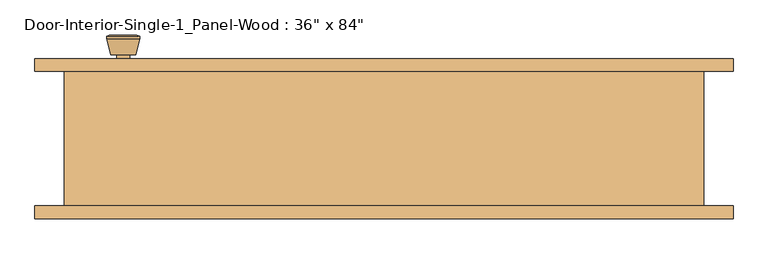
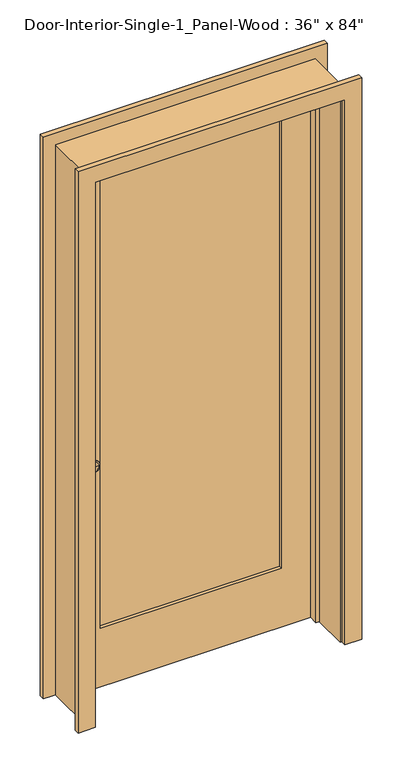
"""IFC4 building model written with IfcOpenShell, lengths in millimetres: door geometry."""

from ifc_helpers import new_model, si_unit, point, frame, frame_2d, origin, place, context, project, spatial, polyline, circle_curve, trimmed, segment, composite_curve, outline, extrude, faceted_brep, source, transform, mapped, element, save
from ifc_brep_helpers import plane_surface, cylinder_surface, revolved_surface, advanced_brep


def door_9c4ddfbd(model_context):
    return source(origin(), model_context, "Body", "SolidModel", [
        advanced_brep(
        [(-393.7, 57.5, 914.4), (-383.7, 57.5, 914.4), (-403.7, 57.5, 914.4), (-373.2241324, 8.5, 914.4), (-393.7, 8.5, 914.4), (-414.1758676, 8.5, 914.4), (-368.7, 10.3278681, 914.4), (-418.7, 10.3278681, 914.4), (-368.7, 13.7915463, 914.4), (-418.7, 13.7915463, 914.4), (-375.063764, 38.5, 914.4), (-412.336236, 38.5, 914.4), (-383.7, 38.5, 914.4), (-403.7, 38.5, 914.4)],
        [
            (0, 1),
            (1, 2, circle_curve(frame((-393.7, 57.5, 914.4), z_axis=(0.0, 1.0, 0.0), x_axis=(-1.0, 0.0, 0.0)), 10.0)),
            (2, 0),
            (2, 1, circle_curve(frame((-393.7, 57.5, 914.4), z_axis=(0.0, 1.0, 0.0), x_axis=(-1.0, 0.0, 0.0)), 10.0)),
            (3, 4),
            (4, 5),
            (5, 3, circle_curve(frame((-393.7, 8.5, 914.4), z_axis=(0.0, -1.0, 0.0), x_axis=(-1.0, 0.0, 0.0)), 20.4758676)),
            (3, 5, circle_curve(frame((-393.7, 8.5, 914.4), z_axis=(0.0, -1.0, 0.0), x_axis=(-1.0, 0.0, 0.0)), 20.4758676)),
            (6, 3),
            (5, 7),
            (7, 6, circle_curve(frame((-393.7, 10.3278681, 914.4), z_axis=(0.0, -1.0, 0.0), x_axis=(-1.0, 0.0, 0.0)), 25.0)),
            (6, 7, circle_curve(frame((-393.7, 10.3278681, 914.4), z_axis=(0.0, -1.0, 0.0), x_axis=(-1.0, 0.0, 0.0)), 25.0)),
            (8, 6),
            (7, 9),
            (9, 8, circle_curve(frame((-393.7, 13.7915463, 914.4), z_axis=(0.0, -1.0, 0.0), x_axis=(-1.0, 0.0, 0.0)), 25.0)),
            (8, 9, circle_curve(frame((-393.7, 13.7915463, 914.4), z_axis=(0.0, -1.0, 0.0), x_axis=(-1.0, 0.0, 0.0)), 25.0)),
            (10, 8),
            (9, 11),
            (11, 10, circle_curve(frame((-393.7, 38.5, 914.4), z_axis=(0.0, -1.0, 0.0), x_axis=(-1.0, 0.0, 0.0)), 18.636236)),
            (10, 11, circle_curve(frame((-393.7, 38.5, 914.4), z_axis=(0.0, -1.0, 0.0), x_axis=(-1.0, 0.0, 0.0)), 18.636236)),
            (12, 10),
            (11, 13),
            (13, 12, circle_curve(frame((-393.7, 38.5, 914.4), z_axis=(0.0, -1.0, 0.0), x_axis=(-1.0, 0.0, 0.0)), 10.0)),
            (12, 13, circle_curve(frame((-393.7, 38.5, 914.4), z_axis=(0.0, -1.0, 0.0), x_axis=(-1.0, 0.0, 0.0)), 10.0)),
            (1, 12),
            (13, 2),
        ],
        [
            plane_surface(frame((-393.7, 57.5, 914.4), z_axis=(0.0, 1.0, 0.0), x_axis=(-1.0, 0.0, 0.0))),
            plane_surface(frame((-393.7, 8.5, 914.4), z_axis=(0.0, -1.0, 0.0), x_axis=(-1.0, 0.0, 0.0))),
            revolved_surface(polyline([(-414.1758676, 8.5, 914.4), (-418.7, 10.3278681, 914.4)]), (-393.7, 57.5, 914.4), (0.0, 1.0, 0.0)),
            cylinder_surface(frame((-393.7, 57.5, 914.4), z_axis=(0.0, 1.0, 0.0), x_axis=(-1.0, 0.0, 0.0)), 25.0),
            revolved_surface(polyline([(-418.7, 13.7915463, 914.4), (-412.336236, 38.5, 914.4)]), (-393.7, 57.5, 914.4), (0.0, 1.0, 0.0)),
            plane_surface(frame((-393.7, 38.5, 914.4), z_axis=(0.0, 1.0, 0.0), x_axis=(-1.0, 0.0, 0.0))),
            cylinder_surface(frame((-393.7, 57.5, 914.4), z_axis=(0.0, 1.0, 0.0), x_axis=(-1.0, 0.0, 0.0)), 10.0),
        ],
        [
            (0, [[1, 2, 3]]),
            (0, [[-3, 4, -1]]),
            (1, [[5, 6, 7]]),
            (1, [[-6, -5, 8]]),
            (2, [[9, -7, 10, 11]]),
            (2, [[-10, -8, -9, 12]]),
            (3, [[13, -11, 14, 15]]),
            (3, [[-14, -12, -13, 16]]),
            (4, [[17, -15, 18, 19]]),
            (4, [[-18, -16, -17, 20]]),
            (5, [[21, -19, 22, 23]]),
            (5, [[-22, -20, -21, 24]]),
            (6, [[25, -23, 26, -2]]),
            (6, [[-26, -24, -25, -4]]),
        ],
    ),
        extrude(outline(composite_curve([segment(trimmed(circle_curve(frame_2d((914.4, -393.7)), 30.0), [point((914.4, -423.7))], [point((914.4, -363.7))], False, "CARTESIAN"), True, "CONTINUOUS"), segment(trimmed(circle_curve(frame_2d((914.4, -393.7)), 30.0), [point((914.4, -363.7))], [point((914.4, -423.7))], False, "CARTESIAN"), True, "CONTINUOUS")], self_intersect=False)), frame((0.0, 57.5, 0.0), z_axis=(0.0, 1.0, 0.0), x_axis=(0.0, 0.0, 1.0)), (0.0, 0.0, 1.0), 6.0),
        advanced_brep(
        [(-393.7, 104.425, 914.4), (-403.7, 104.425, 914.4), (-383.7, 104.425, 914.4), (-373.2241324, 153.425, 914.4), (-414.1758676, 153.425, 914.4), (-393.7, 153.425, 914.4), (-368.7, 151.5971319, 914.4), (-418.7, 151.5971319, 914.4), (-368.7, 148.1334537, 914.4), (-418.7, 148.1334537, 914.4), (-375.063764, 123.425, 914.4), (-412.336236, 123.425, 914.4), (-383.7, 123.425, 914.4), (-403.7, 123.425, 914.4)],
        [
            (0, 1),
            (1, 2, circle_curve(frame((-393.7, 104.425, 914.4), z_axis=(0.0, -1.0, 0.0), x_axis=(-1.0, 0.0, 0.0)), 10.0)),
            (2, 0),
            (2, 1, circle_curve(frame((-393.7, 104.425, 914.4), z_axis=(0.0, -1.0, 0.0), x_axis=(-1.0, 0.0, 0.0)), 10.0)),
            (3, 4, circle_curve(frame((-393.7, 153.425, 914.4), z_axis=(0.0, 1.0, 0.0), x_axis=(-1.0, 0.0, 0.0)), 20.4758676)),
            (4, 5),
            (5, 3),
            (4, 3, circle_curve(frame((-393.7, 153.425, 914.4), z_axis=(0.0, 1.0, 0.0), x_axis=(-1.0, 0.0, 0.0)), 20.4758676)),
            (6, 7, circle_curve(frame((-393.7, 151.5971319, 914.4), z_axis=(0.0, 1.0, 0.0), x_axis=(-1.0, 0.0, 0.0)), 25.0)),
            (7, 4),
            (3, 6),
            (7, 6, circle_curve(frame((-393.7, 151.5971319, 914.4), z_axis=(0.0, 1.0, 0.0), x_axis=(-1.0, 0.0, 0.0)), 25.0)),
            (8, 9, circle_curve(frame((-393.7, 148.1334537, 914.4), z_axis=(0.0, 1.0, 0.0), x_axis=(-1.0, 0.0, 0.0)), 25.0)),
            (9, 7),
            (6, 8),
            (9, 8, circle_curve(frame((-393.7, 148.1334537, 914.4), z_axis=(0.0, 1.0, 0.0), x_axis=(-1.0, 0.0, 0.0)), 25.0)),
            (10, 11, circle_curve(frame((-393.7, 123.425, 914.4), z_axis=(0.0, 1.0, 0.0), x_axis=(-1.0, 0.0, 0.0)), 18.636236)),
            (11, 9),
            (8, 10),
            (11, 10, circle_curve(frame((-393.7, 123.425, 914.4), z_axis=(0.0, 1.0, 0.0), x_axis=(-1.0, 0.0, 0.0)), 18.636236)),
            (12, 13, circle_curve(frame((-393.7, 123.425, 914.4), z_axis=(0.0, 1.0, 0.0), x_axis=(-1.0, 0.0, 0.0)), 10.0)),
            (13, 11),
            (10, 12),
            (13, 12, circle_curve(frame((-393.7, 123.425, 914.4), z_axis=(0.0, 1.0, 0.0), x_axis=(-1.0, 0.0, 0.0)), 10.0)),
            (1, 13),
            (12, 2),
        ],
        [
            plane_surface(frame((-393.7, 104.425, 914.4), z_axis=(0.0, -1.0, 0.0), x_axis=(-1.0, 0.0, 0.0))),
            plane_surface(frame((-393.7, 153.425, 914.4), z_axis=(0.0, 1.0, 0.0), x_axis=(-1.0, 0.0, 0.0))),
            revolved_surface(polyline([(-414.1758676, 153.425, 914.4), (-418.7, 151.5971319, 914.4)]), (-393.7, 104.425, 914.4), (0.0, -1.0, 0.0)),
            cylinder_surface(frame((-393.7, 104.425, 914.4), z_axis=(0.0, -1.0, 0.0), x_axis=(-1.0, 0.0, 0.0)), 25.0),
            revolved_surface(polyline([(-418.7, 148.1334537, 914.4), (-412.336236, 123.425, 914.4)]), (-393.7, 104.425, 914.4), (0.0, -1.0, 0.0)),
            plane_surface(frame((-393.7, 123.425, 914.4), z_axis=(0.0, -1.0, 0.0), x_axis=(-1.0, 0.0, 0.0))),
            cylinder_surface(frame((-393.7, 104.425, 914.4), z_axis=(0.0, -1.0, 0.0), x_axis=(-1.0, 0.0, 0.0)), 10.0),
        ],
        [
            (0, [[1, 2, 3]]),
            (0, [[-3, 4, -1]]),
            (1, [[5, 6, 7]]),
            (1, [[8, -7, -6]]),
            (2, [[9, 10, -5, 11]]),
            (2, [[12, -11, -8, -10]]),
            (3, [[13, 14, -9, 15]]),
            (3, [[16, -15, -12, -14]]),
            (4, [[17, 18, -13, 19]]),
            (4, [[20, -19, -16, -18]]),
            (5, [[21, 22, -17, 23]]),
            (5, [[24, -23, -20, -22]]),
            (6, [[-2, 25, -21, 26]]),
            (6, [[-4, -26, -24, -25]]),
        ],
    ),
        extrude(outline(composite_curve([segment(trimmed(circle_curve(frame_2d((914.4, -393.7)), 30.0), [point((914.4, -423.7))], [point((914.4, -363.7))], False, "CARTESIAN"), True, "CONTINUOUS"), segment(trimmed(circle_curve(frame_2d((914.4, -393.7)), 30.0), [point((914.4, -363.7))], [point((914.4, -423.7))], False, "CARTESIAN"), True, "CONTINUOUS")], self_intersect=False)), frame((0.0, 98.425, 0.0), z_axis=(0.0, 1.0, 0.0), x_axis=(0.0, 0.0, 1.0)), (0.0, 0.0, 1.0), 6.0),
        faceted_brep([(482.6, 98.425, 0.0), (482.6, -104.775, 0.0), (457.2, -104.775, 0.0), (457.2, 28.575, 0.0), (444.5, 28.575, 0.0), (444.5, 63.5, 0.0), (457.2, 63.5, 0.0), (457.2, 98.425, 0.0), (482.6, 98.425, 2159.0), (482.6, -104.775, 2159.0), (-482.6, -104.775, 2159.0), (-482.6, -104.775, 0.0), (-457.2, -104.775, 0.0), (-457.2, -104.775, 2133.6), (457.2, -104.775, 2133.6), (457.2, 28.575, 2133.6), (-457.2, 28.575, 2133.6), (-457.2, 28.575, 0.0), (-444.5, 28.575, 0.0), (-444.5, 28.575, 2120.9), (444.5, 28.575, 2120.9), (444.5, 63.5, 2120.9), (-444.5, 63.5, 2120.9), (-444.5, 63.5, 0.0), (-457.2, 63.5, 0.0), (-457.2, 63.5, 2133.6), (457.2, 63.5, 2133.6), (457.2, 98.425, 2133.6), (-457.2, 98.425, 2133.6), (-457.2, 98.425, 0.0), (-482.6, 98.425, 0.0), (-482.6, 98.425, 2159.0)], [[[0, 1, 2, 3, 4, 5, 6, 7]], [[1, 0, 8, 9]], [[2, 1, 9, 10, 11, 12, 13, 14]], [[3, 2, 14, 15]], [[4, 3, 15, 16, 17, 18, 19, 20]], [[5, 4, 20, 21]], [[6, 5, 21, 22, 23, 24, 25, 26]], [[7, 6, 26, 27]], [[0, 7, 27, 28, 29, 30, 31, 8]], [[9, 8, 31, 10]], [[15, 14, 13, 16]], [[21, 20, 19, 22]], [[27, 26, 25, 28]], [[30, 29, 24, 23, 18, 17, 12, 11]], [[10, 31, 30, 11]], [[16, 13, 12, 17]], [[22, 19, 18, 23]], [[28, 25, 24, 29]]]),
        extrude(outline(polyline([(2133.6, -457.2), (0.0, -457.2), (0.0, 457.2), (2133.6, 457.2), (2133.6, -457.2)]), holes=[polyline([(2014.5375, -336.55), (2014.5375, 336.55), (231.775, 336.55), (231.775, -336.55), (2014.5375, -336.55)])]), frame((0.0, 63.5, 0.0), z_axis=(0.0, 1.0, 0.0), x_axis=(0.0, 0.0, 1.0)), (0.0, 0.0, 1.0), 34.925),
        extrude(outline(polyline([(336.55, 75.1416667), (-336.55, 75.1416667), (-336.55, 86.7833333), (336.55, 86.7833333), (336.55, 75.1416667)])), frame((0.0, 0.0, 231.775), z_axis=(0.0, 0.0, 1.0), x_axis=(1.0, 0.0, 0.0)), (0.0, 0.0, 1.0), 1782.7625),
        extrude(outline(polyline([(0.0, 463.55), (0.0, 527.05), (2203.45, 527.05), (2203.45, -527.05), (0.0, -527.05), (0.0, -463.55), (2139.95, -463.55), (2139.95, 463.55), (0.0, 463.55)])), frame((0.0, 98.425, 0.0), z_axis=(0.0, 1.0, 0.0), x_axis=(0.0, 0.0, 1.0)), (0.0, 0.0, 1.0), 19.05),
        extrude(outline(polyline([(0.0, 463.55), (0.0, 527.05), (2203.45, 527.05), (2203.45, -527.05), (0.0, -527.05), (0.0, -463.55), (2139.95, -463.55), (2139.95, 463.55), (0.0, 463.55)])), frame((0.0, -123.825, 0.0), z_axis=(0.0, 1.0, 0.0), x_axis=(0.0, 0.0, 1.0)), (0.0, 0.0, 1.0), 19.05),
    ])


if __name__ == "__main__":
    model = new_model("IFC4")
    model_context = context("Model", 3, world=origin())
    ifc_project = project(units=[si_unit("LENGTHUNIT", "METRE", prefix="MILLI")], contexts=[model_context])
    site = spatial("IfcSite", under=ifc_project)
    building = spatial("IfcBuilding", under=site)
    placement = place(None, origin())
    door_shape = door_9c4ddfbd(model_context)
    element("IfcDoor", 1, ObjectType="Door-Interior-Single-1_Panel-Wood : 36\" x 84\"", at=placement, inside=building, context=model_context, shape_type="MappedRepresentation", body=[
        mapped(door_shape, transform((0.0, 0.0, 0.0), x_axis=(1.0, 0.0, 0.0), y_axis=(0.0, 1.0, 0.0), z_axis=(0.0, 0.0, 1.0))),
    ])
    save(model, "model.ifc")

# Revit data of these elements
# Type "Door-Interior-Single-1_Panel-Wood : 36\" x 84\""
#   Type Mark = "8"
#   Assembly Code = "C1020300"
#   Analytic Construction = "Wooden"
#   Top Rail = 0' - 4 11/16"
#   Thickness = 0' - 1 3/8"
#   Thermal Resistance (R) = 2.5876 (h·ft²·°F)/BTU
#   Swing Angle [instance default] = 90.00°
#   Stiles = 0' - 4 3/4"
#   Rough Width = 3' - 2"
#   Rough Height = 7' - 1"
#   Height = 7' - 0"
#   Width = 3' - 0"
#   Heat Transfer Coefficient (U) = 0.3865 BTU/(h·ft²·°F)
#   Bottom Rail = 0' - 9 1/8"
#   Trim Material = Cherry
#   Panel Material = Cherry
#   Frame Material = Cherry
#   Door Handle Material = Aluminum
#   Visual Light Transmittance = 0
#   Solar Heat Gain Coefficient = 0
#   Wall Closure = (empty or 0)
#   Function = (empty or 0)
# Element 1 (IfcDoor, "Door-Interior-Single-1_Panel-Wood : 36\" x 84\"")
#   Materials on its faces: "Cherry", "Aluminum"
# Materials
#   "Cherry": class "Wood", colour RGB 226 177 128, transparency 0, Description = "Prunus Serotina", Cost = 0
#   "Aluminum": class "Metal", colour RGB 247 247 247, transparency 0, Description = "Aluminum 6061", Cost = 0
